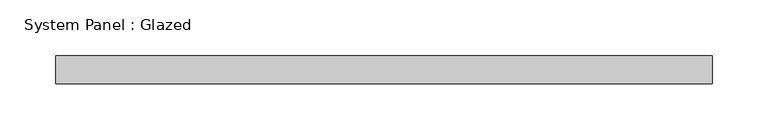
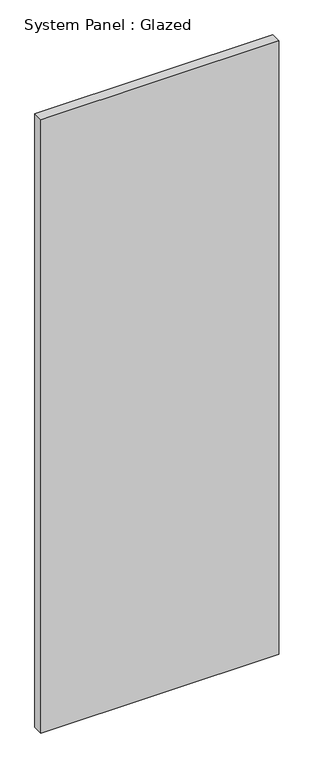
"""IFC4 building model written with IfcOpenShell, lengths in millimetres: plate geometry, System Panel : Glazed."""

from ifc_helpers import new_model, si_unit, origin, origin_with_axes, place, context, project, spatial, polyline, outline, extrude, source, transform, mapped, element, save


def system_panel_glazed_b741adec(model_context):
    return source(origin(), model_context, "Body", "SweptSolid", [
        extrude(outline(polyline([(295.275, 19.05), (-295.275, 19.05), (-295.275, 44.45), (295.275, 44.45), (295.275, 19.05)])), origin_with_axes(), (0.0, 0.0, 1.0), 1609.1531464),
    ])


if __name__ == "__main__":
    model = new_model("IFC4")
    model_context = context("Model", 3, world=origin())
    ifc_project = project(units=[si_unit("LENGTHUNIT", "METRE", prefix="MILLI")], contexts=[model_context])
    site = spatial("IfcSite", under=ifc_project)
    building = spatial("IfcBuilding", under=site)
    placement = place(None, origin())
    system_panel_glazed_shape = system_panel_glazed_b741adec(model_context)
    element("IfcPlate", 1, ObjectType="System Panel : Glazed", at=placement, inside=building, context=model_context, shape_type="MappedRepresentation", body=[
        mapped(system_panel_glazed_shape, transform((0.0, 0.0, 0.0), x_axis=(1.0, 0.0, 0.0), y_axis=(0.0, 1.0, 0.0), z_axis=(0.0, 0.0, 1.0))),
    ])
    save(model, "model.ifc")

# Revit data of these elements
# Type "System Panel : Glazed"
#   Construction Type Id = "GSP4R"
#   Analytic Construction = "1/8 in Pilkington single glazing"
#   Visual Light Transmittance = 0.9
#   Solar Heat Gain Coefficient = 0.86
#   Heat Transfer Coefficient (U) = 1.18115 BTU/(h·ft²·°F)
#   Define Thermal Properties by = 1
# Element 1 (IfcPlate, "System Panel : Glazed")
#   Materials on its faces: "Glass"
# Materials
#   "Glass": class "Glass", colour RGB 0 128 192, transparency 0.75, Description = "Soda Lime Glass", Cost = 0
